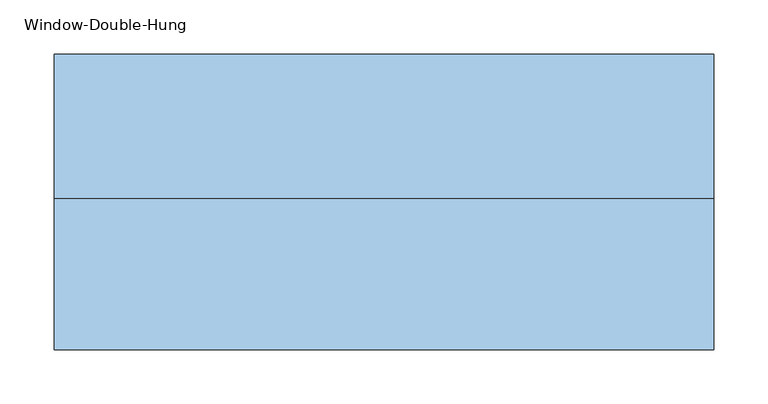
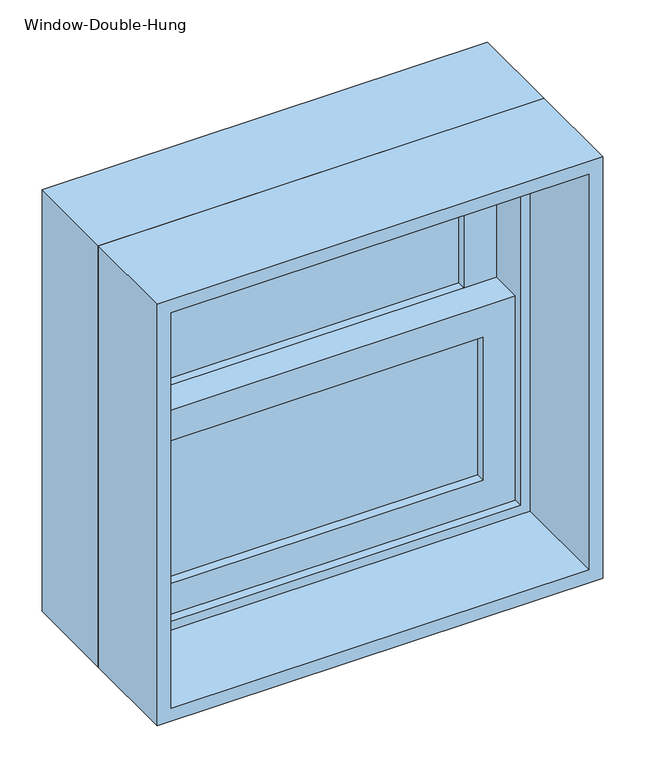
"""IFC4 building model written with IfcOpenShell, lengths in millimetres: window geometry, Window-Double-Hung."""

from ifc_helpers import new_model, si_unit, frame, origin, place, context, project, spatial, polyline, outline, extrude, source, transform, mapped, element, save


def window_double_hung_d0105baa(model_context):
    return source(origin(), model_context, "Body", "SweptSolid", [
        extrude(outline(polyline([(228.6, 57.15), (228.6, 50.8), (-228.6, 50.8), (-228.6, 57.15), (228.6, 57.15)])), frame((0.0, 0.0, 990.6), z_axis=(0.0, 0.0, 1.0), x_axis=(1.0, 0.0, 0.0)), (0.0, 0.0, 1.0), 206.375),
        extrude(outline(polyline([(-228.6, 44.45), (228.6, 44.45), (228.6, 38.1), (-228.6, 38.1), (-228.6, 44.45)])), frame((0.0, 0.0, 990.6), z_axis=(0.0, 0.0, 1.0), x_axis=(1.0, 0.0, 0.0)), (0.0, 0.0, 1.0), 206.375),
        extrude(outline(polyline([(228.6, 101.6), (228.6, 95.25), (-228.6, 95.25), (-228.6, 101.6), (228.6, 101.6)])), frame((0.0, 0.0, 1241.425), z_axis=(0.0, 0.0, 1.0), x_axis=(1.0, 0.0, 0.0)), (0.0, 0.0, 1.0), 206.375),
        extrude(outline(polyline([(-228.6, 88.9), (228.6, 88.9), (228.6, 82.55), (-228.6, 82.55), (-228.6, 88.9)])), frame((0.0, 0.0, 1241.425), z_axis=(0.0, 0.0, 1.0), x_axis=(1.0, 0.0, 0.0)), (0.0, 0.0, 1.0), 206.375),
        extrude(outline(polyline([(1241.425, -273.05), (946.15, -273.05), (946.15, 273.05), (1241.425, 273.05), (1241.425, -273.05)]), holes=[polyline([(1196.975, 228.6), (990.6, 228.6), (990.6, -228.6), (1196.975, -228.6), (1196.975, 228.6)])]), frame((0.0, 25.4, 0.0), z_axis=(0.0, 1.0, 0.0), x_axis=(0.0, 0.0, 1.0)), (0.0, 0.0, 1.0), 44.45),
        extrude(outline(polyline([(1492.25, -273.05), (1196.975, -273.05), (1196.975, 273.05), (1492.25, 273.05), (1492.25, -273.05)]), holes=[polyline([(1447.8, 228.6), (1241.425, 228.6), (1241.425, -228.6), (1447.8, -228.6), (1447.8, 228.6)])]), frame((0.0, 69.85, 0.0), z_axis=(0.0, 1.0, 0.0), x_axis=(0.0, 0.0, 1.0)), (0.0, 0.0, 1.0), 44.45),
        extrude(outline(polyline([(1524.0, -304.8), (914.4, -304.8), (914.4, 304.8), (1524.0, 304.8), (1524.0, -304.8)]), holes=[polyline([(1492.25, 273.05), (946.15, 273.05), (946.15, -273.05), (1492.25, -273.05), (1492.25, 273.05)])]), frame((0.0, 12.7, 0.0), z_axis=(0.0, 1.0, 0.0), x_axis=(0.0, 0.0, 1.0)), (0.0, 0.0, 1.0), 133.35),
        extrude(outline(polyline([(1524.0, 304.8), (1524.0, -304.8), (914.4, -304.8), (914.4, 304.8), (1524.0, 304.8)]), holes=[polyline([(1504.95, 285.75), (933.45, 285.75), (933.45, -285.75), (1504.95, -285.75), (1504.95, 285.75)])]), frame((0.0, -127.0, 0.0), z_axis=(0.0, 1.0, 0.0), x_axis=(0.0, 0.0, 1.0)), (0.0, 0.0, 1.0), 139.7),
    ])


if __name__ == "__main__":
    model = new_model("IFC4")
    model_context = context("Model", 3, world=origin())
    ifc_project = project(units=[si_unit("LENGTHUNIT", "METRE", prefix="MILLI")], contexts=[model_context])
    site = spatial("IfcSite", under=ifc_project)
    building = spatial("IfcBuilding", under=site)
    placement = place(None, origin())
    window_double_hung_shape = window_double_hung_d0105baa(model_context)
    element("IfcWindow", 1, ObjectType="Window-Double-Hung", at=placement, inside=building, context=model_context, shape_type="MappedRepresentation", body=[
        mapped(window_double_hung_shape, transform((0.0, 0.0, 0.0), x_axis=(1.0, 0.0, 0.0), y_axis=(0.0, 1.0, 0.0), z_axis=(0.0, 0.0, 1.0))),
    ])
    save(model, "model.ifc")

# Revit data of these elements
# Type "Window-Double-Hung"
#   Type Mark = "20"
#   Fire Rating = "0.5h"
#   Construction Type Id = "DG-DR"
#   Assembly Code = "B2020100"
#   Analytic Construction = "Double glazing - domestic"
#   Wall Thickness [instance default] = 0' - 6"
#   Window Inset [instance default] = 0' - 0"
#   Visual Light Transmittance = 0.81
#   Thermal Resistance (R) = 1.8146 (h·ft²·°F)/BTU
#   Solar Heat Gain Coefficient = 0.76
#   Muntin Width = 1' - 6"
#   Muntin Height = 0' - 8 1/8"
#   Interior Wall Closure [instance default] = 0' - 1 1/2"
#   Rough Width = 2' - 0 1/2"
#   Rough Height = 2' - 0 1/2"
#   Frame Extension [instance default] = 0' - 1 1/4"
#   Exterior Wall Closure [instance default] = 0' - 0 1/2"
#   Extension Jamb [instance default] = 0' - 1 1/2"
#   Heat Transfer Coefficient (U) = 0.5511 BTU/(h·ft²·°F)
#   Height = 2' - 0"
#   Width = 2' - 0"
#   Top Muntin Visibility = yes
#   Indicator Visibility [instance default] = yes
#   Extension Jamb Visibility [instance default] = yes
#   Interior Trim Visibility [instance default] = yes
#   Exterior Trim Visibility [instance default] = yes
#   Define Thermal Properties by = 1
#   Bottom Muntin Visibility = yes
#   Muntin Pattern = Muntin Pattern_2x2 : Muntin Pattern_2x2
#   Interior Trim Material = Wood - Stained
#   Interior Trim = Trim-Window-Interior-Flat : Picture Frame
#   Exterior Trim Material = Clad - White
#   Exterior Trim = Trim-Window-Exterior-Flat : with Sill
#   Glass Panel Material = Glass
#   Exterior Frame Material = Clad - White
#   Interior Frame Material = Wood - Stained
#   Wall Closure = (empty or 0)
# Element 1 (IfcWindow, "Window-Double-Hung")
#   Wall Thickness = 0' - 10"
#   Extension Jamb = 0' - 5 1/2"
#   Materials on its faces: "Wood - Stained", "Glass", "Clad - White"
# Materials
#   "Wood - Stained": class "Wood", colour RGB 224 178 126, transparency 0, Cost = 0
#   "Clad - White": class "Wood", colour RGB 242 242 238, transparency 0, Cost = 0
#   "Glass": class "Glass", colour RGB 0 128 192, transparency 0.75, Description = "Soda Lime Glass", Cost = 0
